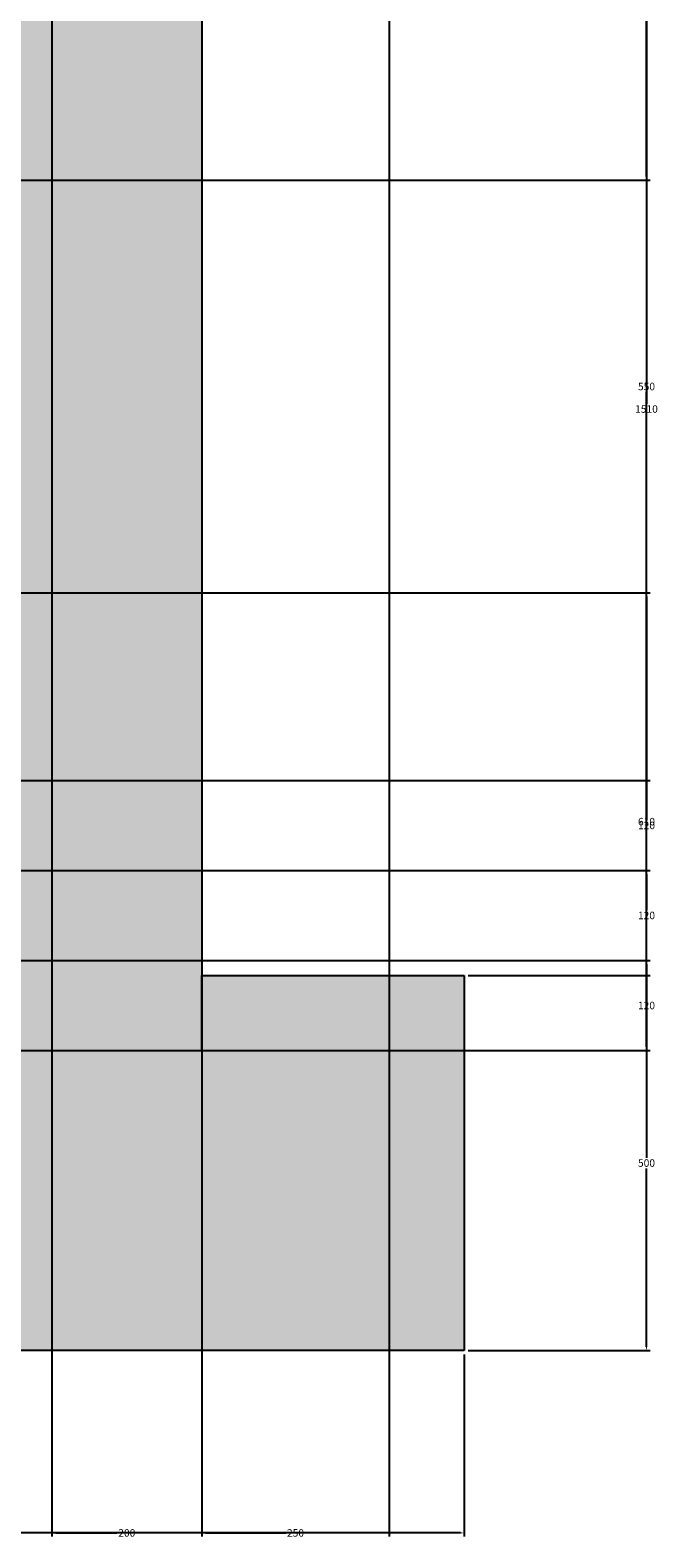
# Model space of a CAD drawing. Units: millimetres. Extents: x 2970 to 7764, y 2196 to 7505.
# Tile 5 of 13: x 6927 to 7764, y 2196 to 4206. Entities that reach past the tile are written whole.
import ezdxf

# ---------------------------------------------------------------- set-up
doc = ezdxf.new("R2010")
doc.units = ezdxf.units.MM
doc.header["$MEASUREMENT"] = 0
for name, color, linetype, lineweight in [('A-ANNO-DIMS', 2, 'Continuous', 18), ('A-ELEV', 7, 'Continuous', 25), ('A-ELEV-PATT', 8, 'Continuous', 13)]:
    doc.layers.add(name, color=color, linetype=linetype, lineweight=lineweight)
doc.styles.get("Standard").update_dxf_attribs({"font": 'arial.ttf'})
doc.dimstyles.get("Standard").update_dxf_attribs({"dimtxt": 10, "dimasz": 5, "dimexe": 5, "dimexo": 5, "dimgap": 2, "dimtad": 0, "dimtih": 1, "dimtoh": 1, "dimdec": 0, "dimzin": 0, "dimdsep": 46, "dimtxsty": 'Standard', "dimcen": 2, "dimadec": 0, "dimazin": 0, "dimtfac": 1, "dimtdec": 0, "dimtofl": 0, "dimtmove": 0, "dimatfit": 3, "dimfxl": 1, "dimtolj": 1, "dimtzin": 0, "dimarcsym": 0})

# ---------------------------------------------------------------- blocks, each defined once
blk = doc.blocks.new('*D10')
at = {"layer": 'A-ANNO-DIMS', "color": 0, "lineweight": -2, "transparency": 16777216}
for p, q in [((3230.5, 2440.8), (3230.5, 2197.8)), ((7505.5, 2440.8), (7505.5, 2197.8)), ((3235.5, 2202.8), (5350.8, 2202.8)), ((7500.5, 2202.8), (5385.2, 2202.8))]:
    blk.add_line(p, q, dxfattribs=at)
at = {"layer": 'A-ANNO-DIMS', "color": 0, "transparency": 16777216}
for points in [[(3235.5, 2203.6), (3235.5, 2202), (3230.5, 2202.8)], [(7500.5, 2203.6), (7500.5, 2202), (7505.5, 2202.8)]]:
    blk.add_solid(points, dxfattribs=at)
at = {"layer": 'Defpoints', "color": 0, "transparency": 16777216}
for p in [(3230.5, 2445.8), (7505.5, 2445.8), (7505.5, 2202.8)]:
    blk.add_point(p, dxfattribs=at)
at = {"layer": 'A-ANNO-DIMS', "color": 0, "transparency": 16777216, "insert": (5368, 2202.8), "char_height": 10, "attachment_point": 5}
blk.add_mtext('\\A1;4275', dxfattribs=at)
blk = doc.blocks.new('*D29')
at = {"layer": 'A-ANNO-DIMS', "color": 0, "lineweight": -2, "transparency": 16777216}
for p, q in [((7510.5, 2945.8), (7753.5, 2945.8)), ((7748.5, 2940.8), (7748.5, 2702.9)), ((7748.5, 2450.8), (7748.5, 2688.7)), ((7510.5, 2445.8), (7753.5, 2445.8))]:
    blk.add_line(p, q, dxfattribs=at)
at = {"layer": 'A-ANNO-DIMS', "color": 0, "transparency": 16777216}
for points in [[(7747.7, 2940.8), (7749.3, 2940.8), (7748.5, 2945.8)], [(7747.7, 2450.8), (7749.3, 2450.8), (7748.5, 2445.8)]]:
    blk.add_solid(points, dxfattribs=at)
at = {"layer": 'Defpoints', "color": 0, "transparency": 16777216}
for p in [(7505.5, 2945.8), (7748.5, 2945.8), (7505.5, 2445.8)]:
    blk.add_point(p, dxfattribs=at)
at = {"layer": 'A-ANNO-DIMS', "color": 0, "transparency": 16777216, "insert": (7748.5, 2695.8), "char_height": 10, "attachment_point": 5}
blk.add_mtext('\\A1;500', dxfattribs=at)
blk = doc.blocks.new('*D30')
at = {"layer": 'A-ANNO-DIMS', "color": 0, "lineweight": -2, "transparency": 16777216}
for p, q in [((7160.5, 4455.8), (7753.5, 4455.8)), ((7748.5, 4450.8), (7748.5, 3707.9)), ((7748.5, 2950.8), (7748.5, 3693.7)), ((7510.5, 2945.8), (7753.5, 2945.8))]:
    blk.add_line(p, q, dxfattribs=at)
at = {"layer": 'A-ANNO-DIMS', "color": 0, "transparency": 16777216}
for points in [[(7747.7, 4450.8), (7749.3, 4450.8), (7748.5, 4455.8)], [(7747.7, 2950.8), (7749.3, 2950.8), (7748.5, 2945.8)]]:
    blk.add_solid(points, dxfattribs=at)
at = {"layer": 'Defpoints', "color": 0, "transparency": 16777216}
for p in [(7155.5, 4455.8), (7748.5, 4455.8), (7505.5, 2945.8)]:
    blk.add_point(p, dxfattribs=at)
at = {"layer": 'A-ANNO-DIMS', "color": 0, "transparency": 16777216, "insert": (7748.5, 3700.8), "char_height": 10, "attachment_point": 5}
blk.add_mtext('\\A1;1510', dxfattribs=at)
blk = doc.blocks.new('*D42')
at = {"layer": 'A-ANNO-DIMS', "color": 0, "lineweight": -2, "transparency": 16777216}
for p, q in [((6955.5, 4450.8), (6955.5, 2197.8)), ((7155.5, 4450.8), (7155.5, 2197.8)), ((6960.5, 2202.8), (7042.4, 2202.8)), ((7150.5, 2202.8), (7068.6, 2202.8))]:
    blk.add_line(p, q, dxfattribs=at)
at = {"layer": 'A-ANNO-DIMS', "color": 0, "transparency": 16777216}
for points in [[(6960.5, 2203.6), (6960.5, 2202), (6955.5, 2202.8)], [(7150.5, 2203.6), (7150.5, 2202), (7155.5, 2202.8)]]:
    blk.add_solid(points, dxfattribs=at)
at = {"layer": 'Defpoints', "color": 0, "transparency": 16777216}
for p in [(6955.5, 4455.8), (7155.5, 4455.8), (7155.5, 2202.8)]:
    blk.add_point(p, dxfattribs=at)
at = {"layer": 'A-ANNO-DIMS', "color": 0, "transparency": 16777216, "insert": (7055.5, 2202.8), "char_height": 10, "attachment_point": 5}
blk.add_mtext('\\A1;200', dxfattribs=at)
blk = doc.blocks.new('*D43')
at = {"layer": 'A-ANNO-DIMS', "color": 0, "lineweight": -2, "transparency": 16777216}
for p, q in [((4355.5, 2840.8), (4355.5, 2197.8)), ((7155.5, 2840.8), (7155.5, 2197.8)), ((4360.5, 2202.8), (5738.5, 2202.8)), ((7150.5, 2202.8), (5772.5, 2202.8))]:
    blk.add_line(p, q, dxfattribs=at)
at = {"layer": 'A-ANNO-DIMS', "color": 0, "transparency": 16777216}
for points in [[(4360.5, 2203.6), (4360.5, 2202), (4355.5, 2202.8)], [(7150.5, 2203.6), (7150.5, 2202), (7155.5, 2202.8)]]:
    blk.add_solid(points, dxfattribs=at)
at = {"layer": 'Defpoints', "color": 0, "transparency": 16777216}
for p in [(4355.5, 2845.8), (7155.5, 2845.8), (7155.5, 2202.8)]:
    blk.add_point(p, dxfattribs=at)
at = {"layer": 'A-ANNO-DIMS', "color": 0, "transparency": 16777216, "insert": (5755.5, 2202.8), "char_height": 10, "attachment_point": 5}
blk.add_mtext('\\A1;2800', dxfattribs=at)
blk = doc.blocks.new('*D50')
at = {"layer": 'A-ANNO-DIMS', "color": 0, "lineweight": -2, "transparency": 16777216}
for p, q in [((6760.3, 3455.8), (7753.5, 3455.8)), ((7748.5, 3450.8), (7748.5, 3157.9)), ((7748.5, 2850.8), (7748.5, 3143.7)), ((7160.5, 2845.8), (7753.5, 2845.8))]:
    blk.add_line(p, q, dxfattribs=at)
at = {"layer": 'A-ANNO-DIMS', "color": 0, "transparency": 16777216}
for points in [[(7747.7, 3450.8), (7749.3, 3450.8), (7748.5, 3455.8)], [(7747.7, 2850.8), (7749.3, 2850.8), (7748.5, 2845.8)]]:
    blk.add_solid(points, dxfattribs=at)
at = {"layer": 'Defpoints', "color": 0, "transparency": 16777216}
for p in [(6755.3, 3455.8), (7748.5, 3455.8), (7155.5, 2845.8)]:
    blk.add_point(p, dxfattribs=at)
at = {"layer": 'A-ANNO-DIMS', "color": 0, "transparency": 16777216, "insert": (7748.5, 3150.8), "char_height": 10, "attachment_point": 5}
blk.add_mtext('\\A1;610', dxfattribs=at)
blk = doc.blocks.new('*D51')
at = {"layer": 'A-ANNO-DIMS', "color": 0, "lineweight": -2, "transparency": 16777216}
for p, q in [((6760.3, 4005.8), (7753.5, 4005.8)), ((7748.5, 4000.8), (7748.5, 3737.9)), ((7748.5, 3460.8), (7748.5, 3723.7)), ((6760.3, 3455.8), (7753.5, 3455.8))]:
    blk.add_line(p, q, dxfattribs=at)
at = {"layer": 'A-ANNO-DIMS', "color": 0, "transparency": 16777216}
for points in [[(7747.7, 4000.8), (7749.3, 4000.8), (7748.5, 4005.8)], [(7747.7, 3460.8), (7749.3, 3460.8), (7748.5, 3455.8)]]:
    blk.add_solid(points, dxfattribs=at)
at = {"layer": 'Defpoints', "color": 0, "transparency": 16777216}
for p in [(6755.3, 4005.8), (7748.5, 4005.8), (6755.3, 3455.8)]:
    blk.add_point(p, dxfattribs=at)
at = {"layer": 'A-ANNO-DIMS', "color": 0, "transparency": 16777216, "insert": (7748.5, 3730.8), "char_height": 10, "attachment_point": 5}
blk.add_mtext('\\A1;550', dxfattribs=at)
blk = doc.blocks.new('*D52')
at = {"layer": 'A-ANNO-DIMS', "color": 0, "lineweight": -2, "transparency": 16777216}
for p, q in [((7160.5, 4455.8), (7753.5, 4455.8)), ((7748.5, 4450.8), (7748.5, 4237.9)), ((7748.5, 4010.8), (7748.5, 4223.7)), ((6760.3, 4005.8), (7753.5, 4005.8))]:
    blk.add_line(p, q, dxfattribs=at)
at = {"layer": 'A-ANNO-DIMS', "color": 0, "transparency": 16777216}
for points in [[(7747.7, 4450.8), (7749.3, 4450.8), (7748.5, 4455.8)], [(7747.7, 4010.8), (7749.3, 4010.8), (7748.5, 4005.8)]]:
    blk.add_solid(points, dxfattribs=at)
at = {"layer": 'Defpoints', "color": 0, "transparency": 16777216}
for p in [(7155.5, 4455.8), (7748.5, 4455.8), (6755.3, 4005.8)]:
    blk.add_point(p, dxfattribs=at)
at = {"layer": 'A-ANNO-DIMS', "color": 0, "transparency": 16777216, "insert": (7748.5, 4230.8), "char_height": 10, "attachment_point": 5}
blk.add_mtext('\\A1;450', dxfattribs=at)
blk = doc.blocks.new('*D53')
at = {"layer": 'A-ANNO-DIMS', "color": 0, "lineweight": -2, "transparency": 16777216}
for p, q in [((6910.5, 2965.8), (7753.5, 2965.8)), ((7748.5, 2960.8), (7748.5, 2912.9)), ((7748.5, 2850.8), (7748.5, 2898.7)), ((6910.5, 2845.8), (7753.5, 2845.8))]:
    blk.add_line(p, q, dxfattribs=at)
at = {"layer": 'A-ANNO-DIMS', "color": 0, "transparency": 16777216}
for points in [[(7747.7, 2960.8), (7749.3, 2960.8), (7748.5, 2965.8)], [(7747.7, 2850.8), (7749.3, 2850.8), (7748.5, 2845.8)]]:
    blk.add_solid(points, dxfattribs=at)
at = {"layer": 'Defpoints', "color": 0, "transparency": 16777216}
for p in [(6905.5, 2965.8), (7748.5, 2965.8), (6905.5, 2845.8)]:
    blk.add_point(p, dxfattribs=at)
at = {"layer": 'A-ANNO-DIMS', "color": 0, "transparency": 16777216, "insert": (7748.5, 2905.8), "char_height": 10, "attachment_point": 5}
blk.add_mtext('\\A1;120', dxfattribs=at)
blk = doc.blocks.new('*D54')
at = {"layer": 'A-ANNO-DIMS', "color": 0, "lineweight": -2, "transparency": 16777216}
for p, q in [((6910.5, 3085.8), (7753.5, 3085.8)), ((7748.5, 3080.8), (7748.5, 3032.9)), ((7748.5, 2970.8), (7748.5, 3018.7)), ((6910.5, 2965.8), (7753.5, 2965.8))]:
    blk.add_line(p, q, dxfattribs=at)
at = {"layer": 'A-ANNO-DIMS', "color": 0, "transparency": 16777216}
for points in [[(7747.7, 3080.8), (7749.3, 3080.8), (7748.5, 3085.8)], [(7747.7, 2970.8), (7749.3, 2970.8), (7748.5, 2965.8)]]:
    blk.add_solid(points, dxfattribs=at)
at = {"layer": 'Defpoints', "color": 0, "transparency": 16777216}
for p in [(6905.5, 3085.8), (7748.5, 3085.8), (6905.5, 2965.8)]:
    blk.add_point(p, dxfattribs=at)
at = {"layer": 'A-ANNO-DIMS', "color": 0, "transparency": 16777216, "insert": (7748.5, 3025.8), "char_height": 10, "attachment_point": 5}
blk.add_mtext('\\A1;120', dxfattribs=at)
blk = doc.blocks.new('*D55')
at = {"layer": 'A-ANNO-DIMS', "color": 0, "lineweight": -2, "transparency": 16777216}
for p, q in [((6910.5, 3205.8), (7753.5, 3205.8)), ((7748.5, 3200.8), (7748.5, 3152.9)), ((7748.5, 3090.8), (7748.5, 3138.7)), ((6910.5, 3085.8), (7753.5, 3085.8))]:
    blk.add_line(p, q, dxfattribs=at)
at = {"layer": 'A-ANNO-DIMS', "color": 0, "transparency": 16777216}
for points in [[(7747.7, 3200.8), (7749.3, 3200.8), (7748.5, 3205.8)], [(7747.7, 3090.8), (7749.3, 3090.8), (7748.5, 3085.8)]]:
    blk.add_solid(points, dxfattribs=at)
at = {"layer": 'Defpoints', "color": 0, "transparency": 16777216}
for p in [(6905.5, 3205.8), (7748.5, 3205.8), (6905.5, 3085.8)]:
    blk.add_point(p, dxfattribs=at)
at = {"layer": 'A-ANNO-DIMS', "color": 0, "transparency": 16777216, "insert": (7748.5, 3145.8), "char_height": 10, "attachment_point": 5}
blk.add_mtext('\\A1;120', dxfattribs=at)
blk = doc.blocks.new('*D59')
at = {"layer": 'A-ANNO-DIMS', "color": 0, "lineweight": -2, "transparency": 16777216}
for p, q in [((6005.5, 5250.8), (6005.5, 2197.8)), ((7155.5, 5250.8), (7155.5, 2197.8)), ((6010.5, 2202.8), (6564.1, 2202.8)), ((7150.5, 2202.8), (6596.9, 2202.8))]:
    blk.add_line(p, q, dxfattribs=at)
at = {"layer": 'A-ANNO-DIMS', "color": 0, "transparency": 16777216}
for points in [[(6010.5, 2203.6), (6010.5, 2202), (6005.5, 2202.8)], [(7150.5, 2203.6), (7150.5, 2202), (7155.5, 2202.8)]]:
    blk.add_solid(points, dxfattribs=at)
at = {"layer": 'Defpoints', "color": 0, "transparency": 16777216}
for p in [(6005.5, 5255.8), (7155.5, 5255.8), (7155.5, 2202.8)]:
    blk.add_point(p, dxfattribs=at)
at = {"layer": 'A-ANNO-DIMS', "color": 0, "transparency": 16777216, "insert": (6580.5, 2202.8), "char_height": 10, "attachment_point": 5}
blk.add_mtext('\\A1;1150', dxfattribs=at)
blk = doc.blocks.new('*D60')
at = {"layer": 'A-ANNO-DIMS', "color": 0, "lineweight": -2, "transparency": 16777216}
for p, q in [((7155.5, 5250.8), (7155.5, 2197.8)), ((7405.5, 5000.8), (7405.5, 2197.8)), ((7160.5, 2202.8), (7267.4, 2202.8)), ((7400.5, 2202.8), (7293.6, 2202.8))]:
    blk.add_line(p, q, dxfattribs=at)
at = {"layer": 'A-ANNO-DIMS', "color": 0, "transparency": 16777216}
for points in [[(7160.5, 2203.6), (7160.5, 2202), (7155.5, 2202.8)], [(7400.5, 2203.6), (7400.5, 2202), (7405.5, 2202.8)]]:
    blk.add_solid(points, dxfattribs=at)
at = {"layer": 'Defpoints', "color": 0, "transparency": 16777216}
for p in [(7155.5, 5255.8), (7405.5, 5005.8), (7405.5, 2202.8)]:
    blk.add_point(p, dxfattribs=at)
at = {"layer": 'A-ANNO-DIMS', "color": 0, "transparency": 16777216, "insert": (7280.5, 2202.8), "char_height": 10, "attachment_point": 5}
blk.add_mtext('\\A1;250', dxfattribs=at)

msp = doc.modelspace()

# ---------------------------------------------------------------- hatches: boundary and pattern name
at = {"layer": 'A-ELEV-PATT'}
h = msp.add_hatch(color=256, dxfattribs=at)
h.dxf.hatch_style = 1
h.paths.add_polyline_path([(6405.5, 7255.789), (4305.5, 7255.789), (4305.5, 6505.789), (3730.5, 6505.789), (3730.5, 4205.789), (3730.5, 2945.789), (3730.5, 2895.789), (3830.5, 2895.789), (3830.5, 4205.789), (3830.5, 6405.789), (4405.5, 6405.789), (4405.5, 4205.789), (6905.5, 4205.789), (6905.5, 2945.789), (6905.5, 2845.789), (7155.5, 2845.789), (7155.5, 2945.789), (7155.5, 4205.789), (7155.5, 4455.789), (4555.5, 4455.789), (4555.5, 6505.789), (4555.5, 7005.789), (6155.5, 7005.789), (6155.5, 6755.789), (6405.5, 6755.789)])
h.paths.add_polyline_path([(7405.5, 6755.789), (6155.5, 6755.789), (5755.5, 6755.789), (5755.5, 5005.789), (7405.5, 5005.789)])
h.paths.add_polyline_path([(7155.5, 6505.789), (7155.5, 5255.789), (6005.5, 5255.789), (6005.5, 6505.789)], flags=16)
h.paths.add_polyline_path([(6105.5, 5520.789), (6105.5, 6055.789), (6455.5, 6055.789), (6455.5, 5520.789), (6655.5, 5520.789), (6655.5, 5605.789), (6655.5, 5955.789), (6955.5, 5955.789), (6955.5, 5605.789), (6955.5, 5520.789)], flags=0)
h.paths.add_polyline_path([(6425.5, 5755.789), (6425.5, 5655.789), (6425.5, 5555.789), (6405.5, 5555.789), (6405.5, 5755.789)], flags=0)
h.paths.add_polyline_path([(6955.5, 5505.789), (6955.5, 5405.789), (6655.5, 5405.789), (6655.5, 5505.789)], flags=0)
h = msp.add_hatch(color=256, dxfattribs=at)
h.dxf.hatch_style = 1
h.paths.add_polyline_path([(7505.5, 2945.789), (7155.5, 2945.789), (7155.5, 2845.789), (6905.5, 2845.789), (4355.5, 2845.789), (4355.5, 2895.789), (3730.5, 2895.789), (3730.5, 2945.789), (3230.5, 2945.789), (3230.5, 2445.789), (7505.5, 2445.789)])

# ---------------------------------------------------------------- linework, layer by layer
at = {"layer": 'A-ELEV'}
for p, q in [((7155.5, 4455.789), (7155.5, 4205.789)), ((7155.5, 4205.789), (7155.5, 2945.789)), ((7155.5, 2945.789), (7505.5, 2945.789)), ((7155.5, 2845.789), (7155.5, 2945.789)), ((7505.5, 2945.789), (7505.5, 2445.789)), ((6905.5, 2845.789), (7155.5, 2845.789)), ((7505.5, 2445.789), (3230.5, 2445.789))]:
    msp.add_line(p, q, dxfattribs=at)

# ---------------------------------------------------------------- dimensions: what is measured, and where the dimension line sits
at = {"layer": 'A-ANNO-DIMS'}
for base, p1, p2, picture, middle in [((7155.5, 2202.789), (6005.5, 5255.789), (7155.5, 5255.789), '*D59', (6580.5, 2202.789)), ((7405.5, 2202.789), (7155.5, 5255.789), (7405.5, 5005.789), '*D60', (7280.5, 2202.789)), ((7155.5, 2202.789), (6955.5, 4455.789), (7155.5, 4455.789), '*D42', (7055.5, 2202.789)), ((7155.5, 2202.789), (4355.5, 2845.789), (7155.5, 2845.789), '*D43', (5755.5, 2202.789)), ((7505.5, 2202.789), (3230.5, 2445.789), (7505.5, 2445.789), '*D10', (5368, 2202.789))]:
    dim = msp.add_linear_dim(base=base, p1=p1, p2=p2, dimstyle='Standard', override={"dimdec": 0, "dimlfac": 1, "dimrnd": 0, "dimzin": 0, "dimdsep": 46, "dimlunit": 2}, dxfattribs=at)
    dim.commit()
    dim.dimension.update_dxf_attribs({"geometry": picture, "text_midpoint": middle})
for base, p1, p2, picture, middle in [((7748.5, 4455.789), (6755.271, 4005.789), (7155.5, 4455.789), '*D52', (7748.5, 4230.789)), ((7748.5, 4455.789), (7505.5, 2945.789), (7155.5, 4455.789), '*D30', (7748.5, 3700.789)), ((7748.5, 4005.789), (6755.271, 3455.789), (6755.271, 4005.789), '*D51', (7748.5, 3730.789)), ((7748.5, 3455.789), (7155.5, 2845.789), (6755.271, 3455.789), '*D50', (7748.5, 3150.789)), ((7748.5, 3205.789), (6905.5, 3085.789), (6905.5, 3205.789), '*D55', (7748.5, 3145.789)), ((7748.5, 3085.789), (6905.5, 2965.789), (6905.5, 3085.789), '*D54', (7748.5, 3025.789)), ((7748.5, 2965.789), (6905.5, 2845.789), (6905.5, 2965.789), '*D53', (7748.5, 2905.789)), ((7748.5, 2945.789), (7505.5, 2445.789), (7505.5, 2945.789), '*D29', (7748.5, 2695.789))]:
    dim = msp.add_linear_dim(base=base, p1=p1, p2=p2, angle=90, dimstyle='Standard', override={"dimdec": 0, "dimlfac": 1, "dimrnd": 0, "dimzin": 0, "dimdsep": 46, "dimlunit": 2}, dxfattribs=at)
    dim.commit()
    dim.dimension.update_dxf_attribs({"geometry": picture, "text_midpoint": middle})

doc.saveas('drawing.dxf')
